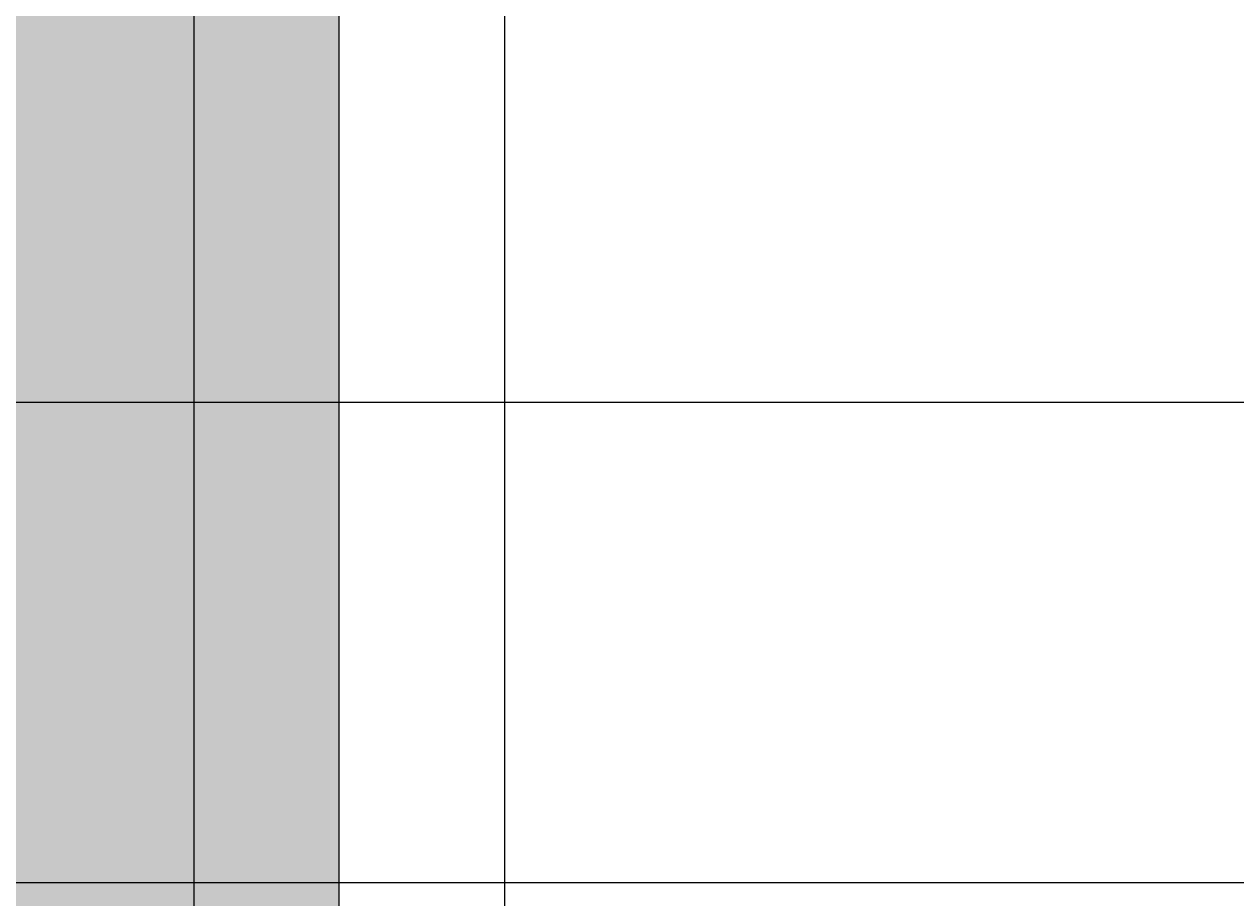
# Model space of a CAD drawing. Units: inches. Extents: x 35362 to 73946, y 43607 to 67532.
# Tile 63 of 134: x 47763 to 49302, y 47689 to 48798. Entities that reach past the tile are written whole.
import ezdxf

# ---------------------------------------------------------------- set-up
doc = ezdxf.new("R2010")
doc.units = ezdxf.units.IN
doc.header["$MEASUREMENT"] = 0
for name, color, linetype, lineweight in [('A-ANNO-DIMS', 2, 'Continuous', 18), ('E-SYMB', 1, 'Continuous', 25), ('E-SYMB-PATT', 1, 'Continuous', 13)]:
    doc.layers.add(name, color=color, linetype=linetype, lineweight=lineweight)
doc.styles.get("Standard").update_dxf_attribs({"font": 'arial.ttf'})
doc.dimstyles.get("Standard").update_dxf_attribs({"dimtxt": 0.18, "dimasz": 0.18, "dimexe": 0.18, "dimexo": 0.0625, "dimgap": 0.09, "dimtad": 0, "dimtih": 1, "dimtoh": 1, "dimdec": 4, "dimzin": 0, "dimdsep": 46, "dimtxsty": 'Standard', "dimcen": 0.09, "dimadec": 0, "dimazin": 0, "dimtfac": 1, "dimtdec": 4, "dimtofl": 0, "dimtmove": 0, "dimatfit": 3, "dimfxl": 1, "dimtolj": 1, "dimtzin": 0, "dimarcsym": 0})

# ---------------------------------------------------------------- blocks, each defined once
blk = doc.blocks.new('*D11')
at = {"layer": 'A-ANNO-DIMS', "color": 0, "lineweight": -2, "transparency": 16777216}
for p, q in [((47978.7, 56028.8), (47978.7, 43606.7)), ((53109.8, 56028.8), (53109.8, 43606.7)), ((47978.8, 43606.9), (50543.9, 43606.9)), ((53109.6, 43606.9), (50544.6, 43606.9))]:
    blk.add_line(p, q, dxfattribs=at)
at = {"layer": 'A-ANNO-DIMS', "color": 0, "transparency": 16777216}
for points in [[(47978.8, 43606.9), (47978.8, 43606.8), (47978.7, 43606.9)], [(53109.6, 43606.9), (53109.6, 43606.8), (53109.8, 43606.9)]]:
    blk.add_solid(points, dxfattribs=at)
at = {"layer": 'Defpoints', "color": 0, "transparency": 16777216}
for p in [(47978.7, 56028.8), (53109.8, 56028.8), (53109.8, 43606.9)]:
    blk.add_point(p, dxfattribs=at)
at = {"layer": 'A-ANNO-DIMS', "color": 0, "transparency": 16777216, "insert": (50544.2, 43606.9), "char_height": 0.18, "attachment_point": 5}
blk.add_mtext('\\A1;5131', dxfattribs=at)
blk = doc.blocks.new('*D13')
at = {"layer": 'A-ANNO-DIMS', "color": 0, "lineweight": -2, "transparency": 16777216}
for p, q in [((48373.5, 51694), (48373.5, 43606.7)), ((51029, 51694), (51029, 43606.7)), ((48373.7, 43606.9), (49700.8, 43606.9)), ((51028.9, 43606.9), (49701.7, 43606.9))]:
    blk.add_line(p, q, dxfattribs=at)
at = {"layer": 'A-ANNO-DIMS', "color": 0, "transparency": 16777216}
for points in [[(48373.7, 43606.9), (48373.7, 43606.8), (48373.5, 43606.9)], [(51028.9, 43606.9), (51028.9, 43606.8), (51029, 43606.9)]]:
    blk.add_solid(points, dxfattribs=at)
at = {"layer": 'Defpoints', "color": 0, "transparency": 16777216}
for p in [(48373.5, 51694.1), (51029, 51694.1), (51029, 43606.9)]:
    blk.add_point(p, dxfattribs=at)
at = {"layer": 'A-ANNO-DIMS', "color": 0, "transparency": 16777216, "insert": (49701.3, 43606.9), "char_height": 0.18, "attachment_point": 5}
blk.add_mtext('\\A1;2655.6', dxfattribs=at)
blk = doc.blocks.new('*D27')
at = {"layer": 'A-ANNO-DIMS', "color": 0, "lineweight": -2, "transparency": 16777216}
for p, q in [((47978.7, 56028.8), (47978.7, 43606.7)), ((48373.5, 53429), (48373.5, 43606.7)), ((47978.8, 43606.9), (48175.7, 43606.9)), ((48373.3, 43606.9), (48176.5, 43606.9))]:
    blk.add_line(p, q, dxfattribs=at)
at = {"layer": 'A-ANNO-DIMS', "color": 0, "transparency": 16777216}
for points in [[(47978.8, 43606.9), (47978.8, 43606.8), (47978.7, 43606.9)], [(48373.3, 43606.9), (48373.3, 43606.8), (48373.5, 43606.9)]]:
    blk.add_solid(points, dxfattribs=at)
at = {"layer": 'Defpoints', "color": 0, "transparency": 16777216}
for p in [(47978.7, 56028.8), (48373.5, 53429), (48373.5, 43606.9)]:
    blk.add_point(p, dxfattribs=at)
at = {"layer": 'A-ANNO-DIMS', "color": 0, "transparency": 16777216, "insert": (48176.1, 43606.9), "char_height": 0.18, "attachment_point": 5}
blk.add_mtext('\\A1;394.8', dxfattribs=at)
blk = doc.blocks.new('*D67')
at = {"layer": 'A-ANNO-DIMS', "color": 0, "lineweight": -2, "transparency": 16777216}
for p, q in [((56873.5, 53351.5), (35361.8, 53351.5)), ((35361.9, 53351.3), (35361.9, 49400.9)), ((35361.9, 45450.1), (35361.9, 49400.5)), ((53793.6, 45449.9), (35361.8, 45449.9))]:
    blk.add_line(p, q, dxfattribs=at)
at = {"layer": 'A-ANNO-DIMS', "color": 0, "transparency": 16777216}
for points in [[(35361.9, 53351.3), (35362, 53351.3), (35361.9, 53351.5)], [(35361.9, 45450.1), (35362, 45450.1), (35361.9, 45449.9)]]:
    blk.add_solid(points, dxfattribs=at)
at = {"layer": 'Defpoints', "color": 0, "transparency": 16777216}
for p in [(35361.9, 53351.5), (56873.6, 53351.5), (53793.6, 45449.9)]:
    blk.add_point(p, dxfattribs=at)
at = {"layer": 'A-ANNO-DIMS', "color": 0, "transparency": 16777216, "insert": (35361.9, 49400.7), "char_height": 0.18, "attachment_point": 5}
blk.add_mtext('\\A1;7901.6', dxfattribs=at)
blk = doc.blocks.new('*D87')
at = {"layer": 'A-ANNO-DIMS', "color": 0, "lineweight": -2, "transparency": 16777216}
for p, q in [((52362.5, 48318.3), (35361.8, 48318.3)), ((35361.9, 48318.1), (35361.9, 47931.4)), ((35361.9, 47544.3), (35361.9, 47931)), ((52362.5, 47544.1), (35361.8, 47544.1))]:
    blk.add_line(p, q, dxfattribs=at)
at = {"layer": 'A-ANNO-DIMS', "color": 0, "transparency": 16777216}
for points in [[(35361.9, 48318.1), (35362, 48318.1), (35361.9, 48318.3)], [(35361.9, 47544.3), (35362, 47544.3), (35361.9, 47544.1)]]:
    blk.add_solid(points, dxfattribs=at)
at = {"layer": 'Defpoints', "color": 0, "transparency": 16777216}
for p in [(35361.9, 48318.3), (52362.6, 48318.3), (52362.6, 47544.1)]:
    blk.add_point(p, dxfattribs=at)
at = {"layer": 'A-ANNO-DIMS', "color": 0, "transparency": 16777216, "insert": (35361.9, 47931.2), "char_height": 0.18, "attachment_point": 5}
blk.add_mtext('\\A1;774.1', dxfattribs=at)
blk = doc.blocks.new('*D89')
at = {"layer": 'A-ANNO-DIMS', "color": 0, "lineweight": -2, "transparency": 16777216}
for p, q in [((53707.7, 48897.7), (35361.8, 48897.7)), ((35361.9, 48897.6), (35361.9, 48303.2)), ((35361.9, 47708.4), (35361.9, 48302.8)), ((53707.7, 47708.2), (35361.8, 47708.2))]:
    blk.add_line(p, q, dxfattribs=at)
at = {"layer": 'A-ANNO-DIMS', "color": 0, "transparency": 16777216}
for points in [[(35361.9, 48897.6), (35362, 48897.6), (35361.9, 48897.7)], [(35361.9, 47708.4), (35362, 47708.4), (35361.9, 47708.2)]]:
    blk.add_solid(points, dxfattribs=at)
at = {"layer": 'Defpoints', "color": 0, "transparency": 16777216}
for p in [(53707.8, 48897.7), (35361.9, 47708.2), (53707.8, 47708.2)]:
    blk.add_point(p, dxfattribs=at)
at = {"layer": 'A-ANNO-DIMS', "color": 0, "transparency": 16777216, "insert": (35361.9, 48303), "char_height": 0.18, "attachment_point": 5}
blk.add_mtext('\\A1;1189.5', dxfattribs=at)

msp = doc.modelspace()

# ---------------------------------------------------------------- hatches: boundary and pattern name
at = {"layer": 'E-SYMB-PATT'}
h = msp.add_hatch(color=256, dxfattribs=at)
h.dxf.hatch_style = 1
h.paths.add_polyline_path([(48163.038, 49689.843), (45390.147, 49689.843), (45390.147, 46919.381), (48163.038, 46919.381)])

# ---------------------------------------------------------------- linework, layer by layer
at = {"layer": 'E-SYMB'}
msp.add_lwpolyline([(45390.147, 49689.843), (48163.038, 49689.843), (48163.038, 46919.381), (45390.147, 46919.381)], close=True, dxfattribs=at)

# ---------------------------------------------------------------- dimensions: what is measured, and where the dimension line sits
at = {"layer": 'A-ANNO-DIMS'}
for base, p1, p2, override, picture, middle in [((53109.76, 43606.859), (47978.665, 56028.836), (53109.76, 56028.836), {"dimdec": 0, "dimlfac": 1, "dimrnd": 0, "dimzin": 0, "dimdsep": 46, "dimlunit": 2}, '*D11', (50544.212, 43606.859)), ((48373.492, 43606.859), (47978.665, 56028.836), (48373.492, 53429.019), {"dimdec": 1, "dimlfac": 1, "dimrnd": 0, "dimzin": 0, "dimdsep": 46, "dimlunit": 2}, '*D27', (48176.078, 43606.859)), ((51029.043, 43606.859), (48373.492, 51694.087), (51029.043, 51694.087), {"dimdec": 1, "dimlfac": 1, "dimrnd": 0, "dimzin": 0, "dimdsep": 46, "dimlunit": 2}, '*D13', (49701.267, 43606.859))]:
    dim = msp.add_linear_dim(base=base, p1=p1, p2=p2, dimstyle='Standard', override=override, dxfattribs=at)
    dim.commit()
    dim.dimension.update_dxf_attribs({"geometry": picture, "text_midpoint": middle})
for base, p1, p2, picture, middle in [((35361.949, 53351.529), (53793.638, 45449.894), (56873.602, 53351.529), '*D67', (35361.949, 49400.712)), ((35361.949, 47708.216), (53707.781, 48897.738), (53707.781, 47708.216), '*D89', (35361.949, 48302.977)), ((35361.949, 48318.269), (52362.557, 47544.134), (52362.557, 48318.269), '*D87', (35361.949, 47931.201))]:
    dim = msp.add_linear_dim(base=base, p1=p1, p2=p2, angle=90, dimstyle='Standard', override={"dimdec": 1, "dimlfac": 1, "dimrnd": 0, "dimzin": 0, "dimdsep": 46, "dimlunit": 2}, dxfattribs=at)
    dim.commit()
    dim.dimension.update_dxf_attribs({"geometry": picture, "text_midpoint": middle})

doc.saveas('drawing.dxf')
